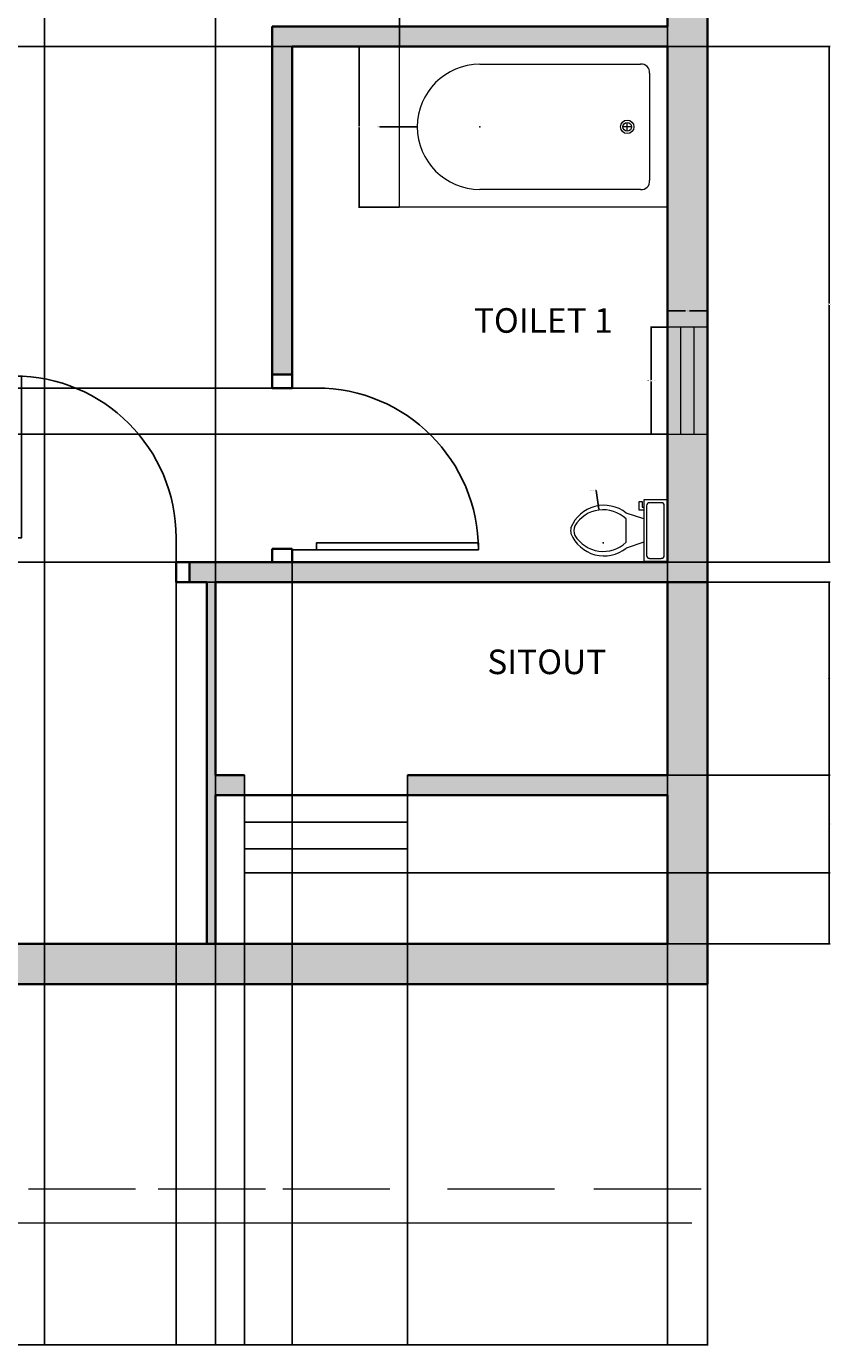
# Model space of a CAD drawing. Units: inches. Extents: x 1839 to 2285, y 722 to 1311.
# Tile 3 of 7: x 2105 to 2285, y 722 to 1018. Entities that reach past the tile are written whole.
import ezdxf

# ---------------------------------------------------------------- set-up
doc = ezdxf.new("R2010")
doc.units = ezdxf.units.IN
for name, color, linetype, lineweight in [('A-ANNO-DIMS', 2, 'Continuous', 18), ('A-AREA-IDEN', 7, 'Continuous', 18), ('A-DOOR', 3, 'Continuous', 25), ('A-FLOR-FIXT', 9, 'Continuous', 18), ('A-FLOR-STRS', 7, 'Continuous', 25), ('A-GLAZ', 4, 'Continuous', 18), ('A-GLAZ-PATT', 9, 'Continuous', 13), ('A-WALL', 7, 'Continuous', 35), ('C-ROAD', 8, 'Continuous', 18)]:
    doc.layers.add(name, color=color, linetype=linetype, lineweight=lineweight)
doc.layers.add('A-WALL-PATT', color=18, linetype='Continuous', lineweight=13, true_color=0x000000)
doc.styles.get("Standard").update_dxf_attribs({"font": 'arial.ttf'})
doc.dimstyles.get("Standard").update_dxf_attribs({"dimtxt": 0.18, "dimasz": 0.18, "dimexe": 0.18, "dimexo": 0.0625, "dimgap": 0.09, "dimtad": 0, "dimtih": 1, "dimtoh": 1, "dimdec": 4, "dimzin": 0, "dimdsep": 46, "dimtxsty": 'Standard', "dimcen": 0.09, "dimadec": 0, "dimazin": 0, "dimtfac": 1, "dimtdec": 4, "dimtofl": 0, "dimtmove": 0, "dimatfit": 3, "dimfxl": 1, "dimtolj": 1, "dimtzin": 0, "dimarcsym": 0})

# ---------------------------------------------------------------- blocks, each defined once
blk = doc.blocks.new('*U3')
for p, q in [((0, 0), (0, -6)), ((-40, 0), (-40, -6))]:
    blk.add_line(p, q)
blk.add_lwpolyline([(0, 0), (0, 40), (-1.75, 40), (-1.75, 0)], close=True)
blk.add_arc((0, 0), 40, 90, 180)
blk = doc.blocks.new('*U5')
for p, q in [((0, 0), (0, -6)), ((40, 0), (40, -6))]:
    blk.add_line(p, q)
blk.add_lwpolyline([(0, 0), (0, 40), (1.75, 40), (1.75, 0)], close=True)
blk.add_arc((0, 0), 40, 0, 90)
blk = doc.blocks.new('Toilet - top')
for p, q in [((9.5, -6), (9.5, -2)), ((-10, -8.5), (-8, -8.5)), ((-10, -9.5), (-10, -8.5)), ((-8, -8.5), (-8, -8)), ((-7, -8), (-7, -9.5)), ((-4, -8), (-6, -14)), ((4, -8), (6, -14)), ((-7, -9.5), (-10, -9.5)), ((4, -14), (-4, -14))]:
    blk.add_line(p, q)
blk.add_lwpolyline([(10.5, -8), (10.5, 0), (-10.5, 0), (-10.5, -8)], close=True)
for points in [[(-9.5, -2), (-9.5, -6)], [(8.5, -1), (-8.5, -1)], [(-8.5, -7), (8.5, -7)]]:
    blk.add_lwpolyline(points)
for centre, radius, start, end in [((-8.62, -1.88), 0.884, 81.8699, 188.1301), ((8.62, -1.88), 0.884, 351.8699, 98.1301), ((-8.62, -6.12), 0.884, 171.8699, 278.1301), ((8.62, -6.12), 0.884, 261.8699, 8.1301), ((3.52, -21.58), 12.17, 141.4691, 247.9714), ((4.2, -21.82), 11.33, 136.3677, 238.9468), ((-3.52, -21.58), 12.17, 292.0284, 38.5307), ((-4.2, -21.82), 11.33, 301.053, 43.6321), ((0, -27.88), 4, 245.7318, 294.2682), ((0, -29), 4, 254.8605, 285.1395)]:
    blk.add_arc(centre, radius, start, end)
blk = doc.blocks.new('Bath Tub - 26 x 60 in.')
for p, q in [((9, -17), (9, -19)), ((8, -18), (10, -18))]:
    blk.add_line(p, q)
blk.add_lwpolyline([(0, -36), (0, 0), (60, 0), (60, -36)], close=True)
for points in [[(6, -4), (42, -4)], [(4, -30), (4, -6)], [(42, -32), (6, -32)]]:
    blk.add_lwpolyline(points)
for radius in [1.5, 1]:
    blk.add_circle((9, -18), radius)
for centre, radius, start, end in [((5.75, -5.75), 1.77, 81.8699, 188.1301), ((42, -18), 14, 270, 90), ((5.75, -30.25), 1.77, 171.8699, 278.1301)]:
    blk.add_arc(centre, radius, start, end)
blk = doc.blocks.new('WIN-24x9')
for p, q in [((3, 0), (3, 24)), ((6, 0), (6, 24))]:
    blk.add_line(p, q)
blk.add_lwpolyline([(0, 24), (0, 0), (9, 0), (9, 24)], close=True)
blk = doc.blocks.new('*D21')
at = {"layer": 'A-ANNO-DIMS', "color": 0, "lineweight": -2, "transparency": 16777216}
for p, q in [((2248.61, 950.49), (2244.9, 950.49)), ((2245.08, 950.31), (2245.08, 938.67)), ((2245.08, 926.67), (2245.08, 938.3)), ((2248.61, 926.49), (2244.9, 926.49))]:
    blk.add_line(p, q, dxfattribs=at)
at = {"layer": 'A-ANNO-DIMS', "color": 0, "transparency": 16777216}
for points in [[(2245.05, 950.31), (2245.11, 950.31), (2245.08, 950.49)], [(2245.05, 926.67), (2245.11, 926.67), (2245.08, 926.49)]]:
    blk.add_solid(points, dxfattribs=at)
at = {"layer": 'Defpoints', "color": 0, "transparency": 16777216}
for p in [(2245.08, 950.49), (2248.68, 950.49), (2248.68, 926.49)]:
    blk.add_point(p, dxfattribs=at)
at = {"layer": 'A-ANNO-DIMS', "color": 0, "transparency": 16777216, "insert": (2245.08, 938.49), "char_height": 0.18, "attachment_point": 5}
blk.add_mtext('\\A1;WINDOW 24 TYP.', dxfattribs=at)
blk = doc.blocks.new('*D22')
at = {"layer": 'A-ANNO-DIMS', "color": 0, "lineweight": -2, "transparency": 16777216}
for p, q in [((2248.68, 950.55), (2248.68, 954.27)), ((2248.86, 954.09), (2252.72, 954.09)), ((2257.5, 954.09), (2253.64, 954.09)), ((2257.68, 950.55), (2257.68, 954.27))]:
    blk.add_line(p, q, dxfattribs=at)
at = {"layer": 'A-ANNO-DIMS', "color": 0, "transparency": 16777216}
for points in [[(2248.86, 954.12), (2248.86, 954.06), (2248.68, 954.09)], [(2257.5, 954.12), (2257.5, 954.06), (2257.68, 954.09)]]:
    blk.add_solid(points, dxfattribs=at)
at = {"layer": 'Defpoints', "color": 0, "transparency": 16777216}
for p in [(2257.68, 954.09), (2248.68, 950.49), (2257.68, 950.49)]:
    blk.add_point(p, dxfattribs=at)
at = {"layer": 'A-ANNO-DIMS', "color": 0, "transparency": 16777216, "insert": (2253.18, 954.09), "char_height": 0.18, "attachment_point": 5}
blk.add_mtext('\\A1;9 TYP.', dxfattribs=at)
blk = doc.blocks.new('*D37')
at = {"layer": 'A-ANNO-DIMS', "color": 0, "lineweight": -2, "transparency": 16777216}
for p, q in [((2188.68, 1013.39), (2188.68, 1022.51)), ((2248.68, 1013.39), (2248.68, 1022.51)), ((2188.86, 1022.33), (2218.17, 1022.33)), ((2248.5, 1022.33), (2219.18, 1022.33))]:
    blk.add_line(p, q, dxfattribs=at)
at = {"layer": 'A-ANNO-DIMS', "color": 0, "transparency": 16777216}
for points in [[(2188.86, 1022.36), (2188.86, 1022.3), (2188.68, 1022.33)], [(2248.5, 1022.36), (2248.5, 1022.3), (2248.68, 1022.33)]]:
    blk.add_solid(points, dxfattribs=at)
at = {"layer": 'Defpoints', "color": 0, "transparency": 16777216}
for p in [(2188.68, 1022.33), (2188.68, 1013.33), (2248.68, 1013.33)]:
    blk.add_point(p, dxfattribs=at)
at = {"layer": 'A-ANNO-DIMS', "color": 0, "transparency": 16777216, "insert": (2218.68, 1022.33), "char_height": 0.18, "attachment_point": 5}
blk.add_mtext('\\A1;TUB 60', dxfattribs=at)
blk = doc.blocks.new('*D38')
at = {"layer": 'A-ANNO-DIMS', "color": 0, "lineweight": -2, "transparency": 16777216}
for p, q in [((2188.61, 1013.33), (2179.5, 1013.33)), ((2179.68, 1013.15), (2179.68, 995.51)), ((2179.68, 977.51), (2179.68, 995.15)), ((2188.61, 977.33), (2179.5, 977.33))]:
    blk.add_line(p, q, dxfattribs=at)
at = {"layer": 'A-ANNO-DIMS', "color": 0, "transparency": 16777216}
for points in [[(2179.65, 1013.15), (2179.71, 1013.15), (2179.68, 1013.33)], [(2179.65, 977.51), (2179.71, 977.51), (2179.68, 977.33)]]:
    blk.add_solid(points, dxfattribs=at)
at = {"layer": 'Defpoints', "color": 0, "transparency": 16777216}
for p in [(2188.68, 1013.33), (2179.68, 977.33), (2188.68, 977.33)]:
    blk.add_point(p, dxfattribs=at)
at = {"layer": 'A-ANNO-DIMS', "color": 0, "transparency": 16777216, "insert": (2179.68, 995.33), "char_height": 0.18, "attachment_point": 5}
blk.add_mtext('\\A1;36', dxfattribs=at)
blk = doc.blocks.new('*D41')
at = {"layer": 'A-ANNO-DIMS', "color": 0, "lineweight": -2, "transparency": 16777216}
for p, q in [((1897.68, 803.27), (1897.68, 722.34)), ((2257.68, 803.27), (2257.68, 722.34)), ((1897.86, 722.52), (2077.39, 722.52)), ((2257.5, 722.52), (2077.97, 722.52))]:
    blk.add_line(p, q, dxfattribs=at)
at = {"layer": 'A-ANNO-DIMS', "color": 0, "transparency": 16777216}
for points in [[(1897.86, 722.55), (1897.86, 722.49), (1897.68, 722.52)], [(2257.5, 722.55), (2257.5, 722.49), (2257.68, 722.52)]]:
    blk.add_solid(points, dxfattribs=at)
at = {"layer": 'Defpoints', "color": 0, "transparency": 16777216}
for p in [(1897.68, 803.33), (2257.68, 803.33), (2257.68, 722.52)]:
    blk.add_point(p, dxfattribs=at)
at = {"layer": 'A-ANNO-DIMS', "color": 0, "transparency": 16777216, "insert": (2077.68, 722.52), "char_height": 0.18, "attachment_point": 5}
blk.add_mtext('\\A1;360', dxfattribs=at)
blk = doc.blocks.new('*D45')
at = {"layer": 'A-ANNO-DIMS', "color": 0, "lineweight": -2, "transparency": 16777216}
for p, q in [((2109.18, 1145.02), (2109.18, 722.34)), ((2248.68, 1142.27), (2248.68, 722.34)), ((2109.36, 722.52), (2178.54, 722.52)), ((2248.5, 722.52), (2179.31, 722.52))]:
    blk.add_line(p, q, dxfattribs=at)
at = {"layer": 'A-ANNO-DIMS', "color": 0, "transparency": 16777216}
for points in [[(2109.36, 722.55), (2109.36, 722.49), (2109.18, 722.52)], [(2248.5, 722.55), (2248.5, 722.49), (2248.68, 722.52)]]:
    blk.add_solid(points, dxfattribs=at)
at = {"layer": 'Defpoints', "color": 0, "transparency": 16777216}
for p in [(2109.18, 1145.08), (2248.68, 1142.33), (2248.68, 722.52)]:
    blk.add_point(p, dxfattribs=at)
at = {"layer": 'A-ANNO-DIMS', "color": 0, "transparency": 16777216, "insert": (2178.93, 722.52), "char_height": 0.18, "attachment_point": 5}
blk.add_mtext('\\A1;139.5', dxfattribs=at)
blk = doc.blocks.new('*D49')
at = {"layer": 'A-ANNO-DIMS', "color": 0, "lineweight": -2, "transparency": 16777216}
for p, q in [((2248.74, 1013.33), (2285.11, 1013.33)), ((2284.93, 1013.15), (2284.93, 955.76)), ((2284.93, 898.01), (2284.93, 955.4)), ((2248.74, 897.83), (2285.11, 897.83))]:
    blk.add_line(p, q, dxfattribs=at)
at = {"layer": 'A-ANNO-DIMS', "color": 0, "transparency": 16777216}
for points in [[(2284.9, 1013.15), (2284.96, 1013.15), (2284.93, 1013.33)], [(2284.9, 898.01), (2284.96, 898.01), (2284.93, 897.83)]]:
    blk.add_solid(points, dxfattribs=at)
at = {"layer": 'Defpoints', "color": 0, "transparency": 16777216}
for p in [(2248.68, 1013.33), (2284.93, 1013.33), (2248.68, 897.83)]:
    blk.add_point(p, dxfattribs=at)
at = {"layer": 'A-ANNO-DIMS', "color": 0, "transparency": 16777216, "insert": (2284.93, 955.58), "char_height": 0.18, "attachment_point": 5}
blk.add_mtext('\\A1;115.5', dxfattribs=at)
blk = doc.blocks.new('*D50')
at = {"layer": 'A-ANNO-DIMS', "color": 0, "lineweight": -2, "transparency": 16777216}
for p, q in [((2145.57, 893.33), (2285.11, 893.33)), ((2284.93, 893.15), (2284.93, 853.01)), ((2284.93, 812.51), (2284.93, 852.65)), ((1906.74, 812.33), (2285.11, 812.33))]:
    blk.add_line(p, q, dxfattribs=at)
at = {"layer": 'A-ANNO-DIMS', "color": 0, "transparency": 16777216}
for points in [[(2284.9, 893.15), (2284.96, 893.15), (2284.93, 893.33)], [(2284.9, 812.51), (2284.96, 812.51), (2284.93, 812.33)]]:
    blk.add_solid(points, dxfattribs=at)
at = {"layer": 'Defpoints', "color": 0, "transparency": 16777216}
for p in [(2145.5, 893.33), (2284.93, 893.33), (1906.68, 812.33)]:
    blk.add_point(p, dxfattribs=at)
at = {"layer": 'A-ANNO-DIMS', "color": 0, "transparency": 16777216, "insert": (2284.93, 852.83), "char_height": 0.18, "attachment_point": 5}
blk.add_mtext('\\A1;81', dxfattribs=at)
blk = doc.blocks.new('*D54')
at = {"layer": 'A-ANNO-DIMS', "color": 0, "lineweight": -2, "transparency": 16777216}
for p, q in [((2164.68, 897.77), (2164.68, 722.34)), ((2248.68, 897.77), (2248.68, 722.34)), ((2164.86, 722.52), (2206.46, 722.52)), ((2248.5, 722.52), (2206.9, 722.52))]:
    blk.add_line(p, q, dxfattribs=at)
at = {"layer": 'A-ANNO-DIMS', "color": 0, "transparency": 16777216}
for points in [[(2164.86, 722.55), (2164.86, 722.49), (2164.68, 722.52)], [(2248.5, 722.55), (2248.5, 722.49), (2248.68, 722.52)]]:
    blk.add_solid(points, dxfattribs=at)
at = {"layer": 'Defpoints', "color": 0, "transparency": 16777216}
for p in [(2164.68, 897.83), (2248.68, 897.83), (2248.68, 722.52)]:
    blk.add_point(p, dxfattribs=at)
at = {"layer": 'A-ANNO-DIMS', "color": 0, "transparency": 16777216, "insert": (2206.68, 722.52), "char_height": 0.18, "attachment_point": 5}
blk.add_mtext('\\A1;84', dxfattribs=at)
blk = doc.blocks.new('*D56')
at = {"layer": 'A-ANNO-DIMS', "color": 0, "lineweight": -2, "transparency": 16777216}
for p, q in [((2147.5, 850.18), (2147.5, 1310.76)), ((2147.68, 1310.58), (2197.64, 1310.58)), ((2248.5, 1310.58), (2198.55, 1310.58)), ((2248.68, 850.18), (2248.68, 1310.76))]:
    blk.add_line(p, q, dxfattribs=at)
at = {"layer": 'A-ANNO-DIMS', "color": 0, "transparency": 16777216}
for points in [[(2147.68, 1310.61), (2147.68, 1310.55), (2147.5, 1310.58)], [(2248.5, 1310.61), (2248.5, 1310.55), (2248.68, 1310.58)]]:
    blk.add_solid(points, dxfattribs=at)
at = {"layer": 'Defpoints', "color": 0, "transparency": 16777216}
for p in [(2248.68, 1310.58), (2147.5, 850.11), (2248.68, 850.11)]:
    blk.add_point(p, dxfattribs=at)
at = {"layer": 'A-ANNO-DIMS', "color": 0, "transparency": 16777216, "insert": (2198.09, 1310.58), "char_height": 0.18, "attachment_point": 5}
blk.add_mtext('\\A1;101.17', dxfattribs=at)
blk = doc.blocks.new('*D57')
at = {"layer": 'A-ANNO-DIMS', "color": 0, "lineweight": -2, "transparency": 16777216}
for p, q in [((2248.74, 893.33), (2285.11, 893.33)), ((2284.93, 893.15), (2284.93, 871.9)), ((2284.93, 850.29), (2284.93, 871.54)), ((2248.74, 850.11), (2285.11, 850.11))]:
    blk.add_line(p, q, dxfattribs=at)
at = {"layer": 'A-ANNO-DIMS', "color": 0, "transparency": 16777216}
for points in [[(2284.9, 893.15), (2284.96, 893.15), (2284.93, 893.33)], [(2284.9, 850.29), (2284.96, 850.29), (2284.93, 850.11)]]:
    blk.add_solid(points, dxfattribs=at)
at = {"layer": 'Defpoints', "color": 0, "transparency": 16777216}
for p in [(2248.68, 893.33), (2284.93, 893.33), (2248.68, 850.11)]:
    blk.add_point(p, dxfattribs=at)
at = {"layer": 'A-ANNO-DIMS', "color": 0, "transparency": 16777216, "insert": (2284.93, 871.72), "char_height": 0.18, "attachment_point": 5}
blk.add_mtext('\\A1;43.22', dxfattribs=at)
blk = doc.blocks.new('*D58')
at = {"layer": 'A-ANNO-DIMS', "color": 0, "lineweight": -2, "transparency": 16777216}
for p, q in [((2102.66, 893.27), (2102.66, 722.34)), ((2138.66, 893.27), (2138.66, 722.34)), ((2102.84, 722.52), (2120.45, 722.52)), ((2138.48, 722.52), (2120.88, 722.52))]:
    blk.add_line(p, q, dxfattribs=at)
at = {"layer": 'A-ANNO-DIMS', "color": 0, "transparency": 16777216}
for points in [[(2102.84, 722.55), (2102.84, 722.49), (2102.66, 722.52)], [(2138.48, 722.55), (2138.48, 722.49), (2138.66, 722.52)]]:
    blk.add_solid(points, dxfattribs=at)
at = {"layer": 'Defpoints', "color": 0, "transparency": 16777216}
for p in [(2102.66, 893.33), (2138.66, 893.33), (2138.66, 722.52)]:
    blk.add_point(p, dxfattribs=at)
at = {"layer": 'A-ANNO-DIMS', "color": 0, "transparency": 16777216, "insert": (2120.66, 722.52), "char_height": 0.18, "attachment_point": 5}
blk.add_mtext('\\A1;36', dxfattribs=at)
blk = doc.blocks.new('*D64')
at = {"layer": 'A-ANNO-DIMS', "color": 0, "lineweight": -2, "transparency": 16777216}
for p, q in [((2248.61, 926.49), (1870.25, 926.49)), ((1870.43, 926.31), (1870.43, 912.34)), ((1870.43, 898.01), (1870.43, 911.98)), ((2248.61, 897.83), (1870.25, 897.83))]:
    blk.add_line(p, q, dxfattribs=at)
at = {"layer": 'A-ANNO-DIMS', "color": 0, "transparency": 16777216}
for points in [[(1870.4, 926.31), (1870.46, 926.31), (1870.43, 926.49)], [(1870.4, 898.01), (1870.46, 898.01), (1870.43, 897.83)]]:
    blk.add_solid(points, dxfattribs=at)
at = {"layer": 'Defpoints', "color": 0, "transparency": 16777216}
for p in [(1870.43, 926.49), (2248.68, 926.49), (2248.68, 897.83)]:
    blk.add_point(p, dxfattribs=at)
at = {"layer": 'A-ANNO-DIMS', "color": 0, "transparency": 16777216, "insert": (1870.43, 912.16), "char_height": 0.18, "attachment_point": 5}
blk.add_mtext('\\A1;28.655', dxfattribs=at)
blk = doc.blocks.new('*D76')
at = {"layer": 'A-ANNO-DIMS', "color": 0, "lineweight": -2, "transparency": 16777216}
for p, q in [((2153.99, 828.2), (2153.99, 722.34)), ((2190.49, 828.2), (2190.49, 722.34)), ((2154.17, 722.52), (2171.91, 722.52)), ((2190.31, 722.52), (2172.56, 722.52))]:
    blk.add_line(p, q, dxfattribs=at)
at = {"layer": 'A-ANNO-DIMS', "color": 0, "transparency": 16777216}
for points in [[(2154.17, 722.55), (2154.17, 722.49), (2153.99, 722.52)], [(2190.31, 722.55), (2190.31, 722.49), (2190.49, 722.52)]]:
    blk.add_solid(points, dxfattribs=at)
at = {"layer": 'Defpoints', "color": 0, "transparency": 16777216}
for p in [(2153.99, 828.26), (2190.49, 828.26), (2190.49, 722.52)]:
    blk.add_point(p, dxfattribs=at)
at = {"layer": 'A-ANNO-DIMS', "color": 0, "transparency": 16777216, "insert": (2172.24, 722.52), "char_height": 0.18, "attachment_point": 5}
blk.add_mtext('\\A1;36.5', dxfattribs=at)
blk = doc.blocks.new('*D77')
at = {"layer": 'A-ANNO-DIMS', "color": 0, "lineweight": -2, "transparency": 16777216}
for p, q in [((2190.55, 850.11), (2285.11, 850.11)), ((2284.93, 849.93), (2284.93, 839.37)), ((2284.93, 828.44), (2284.93, 839.01)), ((2190.55, 828.26), (2285.11, 828.26))]:
    blk.add_line(p, q, dxfattribs=at)
at = {"layer": 'A-ANNO-DIMS', "color": 0, "transparency": 16777216}
for points in [[(2284.9, 849.93), (2284.96, 849.93), (2284.93, 850.11)], [(2284.9, 828.44), (2284.96, 828.44), (2284.93, 828.26)]]:
    blk.add_solid(points, dxfattribs=at)
at = {"layer": 'Defpoints', "color": 0, "transparency": 16777216}
for p in [(2190.49, 850.11), (2284.93, 850.11), (2190.49, 828.26)]:
    blk.add_point(p, dxfattribs=at)
at = {"layer": 'A-ANNO-DIMS', "color": 0, "transparency": 16777216, "insert": (2284.93, 839.19), "char_height": 0.18, "attachment_point": 5}
blk.add_mtext('\\A1;21.85', dxfattribs=at)
blk = doc.blocks.new('*D80')
at = {"layer": 'A-ANNO-DIMS', "color": 0, "lineweight": -2, "transparency": 16777216}
for p, q in [((2147.5, 850.05), (2147.5, 722.34)), ((2153.99, 850.05), (2153.99, 722.34)), ((2147.68, 722.52), (2150.35, 722.52)), ((2153.81, 722.52), (2151.14, 722.52))]:
    blk.add_line(p, q, dxfattribs=at)
at = {"layer": 'A-ANNO-DIMS', "color": 0, "transparency": 16777216}
for points in [[(2147.68, 722.55), (2147.68, 722.49), (2147.5, 722.52)], [(2153.81, 722.55), (2153.81, 722.49), (2153.99, 722.52)]]:
    blk.add_solid(points, dxfattribs=at)
at = {"layer": 'Defpoints', "color": 0, "transparency": 16777216}
for p in [(2147.5, 850.11), (2153.99, 850.11), (2153.99, 722.52)]:
    blk.add_point(p, dxfattribs=at)
at = {"layer": 'A-ANNO-DIMS', "color": 0, "transparency": 16777216, "insert": (2150.74, 722.52), "char_height": 0.18, "attachment_point": 5}
blk.add_mtext('\\A1;6.482', dxfattribs=at)
blk = doc.blocks.new('*D82')
at = {"layer": 'A-ANNO-DIMS', "color": 0, "lineweight": -2, "transparency": 16777216}
for p, q in [((2164.61, 1013.33), (1870.25, 1013.33)), ((1870.43, 1013.15), (1870.43, 975.26)), ((1870.43, 937.01), (1870.43, 974.9)), ((2164.61, 936.83), (1870.25, 936.83))]:
    blk.add_line(p, q, dxfattribs=at)
at = {"layer": 'A-ANNO-DIMS', "color": 0, "transparency": 16777216}
for points in [[(1870.4, 1013.15), (1870.46, 1013.15), (1870.43, 1013.33)], [(1870.4, 937.01), (1870.46, 937.01), (1870.43, 936.83)]]:
    blk.add_solid(points, dxfattribs=at)
at = {"layer": 'Defpoints', "color": 0, "transparency": 16777216}
for p in [(1870.43, 1013.33), (2164.68, 1013.33), (2164.68, 936.83)]:
    blk.add_point(p, dxfattribs=at)
at = {"layer": 'A-ANNO-DIMS', "color": 0, "transparency": 16777216, "insert": (1870.43, 975.08), "char_height": 0.18, "attachment_point": 5}
blk.add_mtext('\\A1;76.5', dxfattribs=at)
blk = doc.blocks.new('*D85')
at = {"layer": 'A-ANNO-DIMS', "color": 0, "lineweight": -2, "transparency": 16777216}
for p, q in [((2184.28, 995.33), (2192.5, 995.33)), ((2206.59, 995.33), (2206.77, 995.33)), ((2206.68, 995.24), (2206.68, 995.42))]:
    blk.add_line(p, q, dxfattribs=at)
at = {"layer": 'A-ANNO-DIMS', "color": 0, "transparency": 16777216}
blk.add_solid([(2192.5, 995.36), (2192.5, 995.3), (2192.68, 995.33)], dxfattribs=at)
at = {"layer": 'Defpoints', "color": 0, "transparency": 16777216}
for p in [(2192.68, 995.33), (2206.68, 995.33)]:
    blk.add_point(p, dxfattribs=at)
at = {"layer": 'A-ANNO-DIMS', "color": 0, "transparency": 16777216, "insert": (2183.97, 995.33), "char_height": 0.18, "attachment_point": 5}
blk.add_mtext('\\A1;R14', dxfattribs=at)
blk = doc.blocks.new('*D92')
at = {"layer": 'A-ANNO-DIMS', "color": 0, "lineweight": -2, "transparency": 16777216}
for p, q in [((2232.56, 913.91), (2232.74, 913.91)), ((2232.74, 913.91), (2233.31, 909.68)), ((2234.23, 902.15), (2234.41, 902.15)), ((2234.32, 902.06), (2234.32, 902.24))]:
    blk.add_line(p, q, dxfattribs=at)
at = {"layer": 'A-ANNO-DIMS', "color": 0, "transparency": 16777216}
blk.add_solid([(2233.34, 909.68), (2233.28, 909.67), (2233.33, 909.5)], dxfattribs=at)
at = {"layer": 'Defpoints', "color": 0, "transparency": 16777216}
for p in [(2233.33, 909.5), (2234.32, 902.15)]:
    blk.add_point(p, dxfattribs=at)
at = {"layer": 'A-ANNO-DIMS', "color": 0, "transparency": 16777216, "insert": (2231.88, 913.91), "char_height": 0.18, "attachment_point": 5}
blk.add_mtext('\\A1;4X R7.419', dxfattribs=at)

msp = doc.modelspace()

# ---------------------------------------------------------------- hatches: boundary and pattern name
at = {"layer": 'A-GLAZ-PATT'}
h = msp.add_hatch(color=256, dxfattribs=at)
h.dxf.hatch_style = 1
h.set_gradient(color1=(0, 0, 255), color2=(255, 255, 0))
h.paths.add_polyline_path([(2251.6771, 950.4862), (2248.6771, 950.4862), (2248.6771, 926.4862), (2251.6771, 926.4862)])
h.paths.add_polyline_path([(2254.6771, 950.4862), (2251.6771, 950.4862), (2251.6771, 926.4862), (2254.6771, 926.4862)])
h.paths.add_polyline_path([(2257.6771, 950.4862), (2254.6771, 950.4862), (2254.6771, 926.4862), (2257.6771, 926.4862)])
at = {"layer": 'A-WALL-PATT'}
h = msp.add_hatch(color=256, dxfattribs=at)
h.dxf.hatch_style = 1
h.paths.add_polyline_path([(1906.6771, 1274.3314), (1942.6771, 1274.3314), (1942.6771, 1283.3314), (1897.6771, 1283.3314), (1897.6771, 968.2107), (1906.6771, 968.2107), (1906.6771, 1013.3314), (1939.6771, 1013.3314), (1939.6771, 1017.8314), (1906.6771, 1017.8314), (1906.6771, 1137.8314), (2050.6771, 1137.8314), (2050.6771, 1142.3314), (1906.6771, 1142.3314)])
h.paths.add_polyline_path([(2064.0508, 1283.3314), (1978.6771, 1283.3314), (1978.6771, 1274.3314), (2050.6771, 1274.3314), (2050.6771, 1184.3314), (2055.1771, 1184.3314), (2055.1771, 1214.3314), (2058.1771, 1214.3314), (2058.1771, 1218.8314), (2055.1771, 1218.8314), (2055.1771, 1274.3314), (2064.0508, 1274.3314)])
h.paths.add_polyline_path([(2182.6416, 1283.3314), (2088.0508, 1283.3314), (2088.0508, 1274.3314), (2104.6771, 1274.3314), (2104.6771, 1218.8314), (2094.1771, 1218.8314), (2094.1771, 1214.3314), (2104.6771, 1214.3314), (2104.6771, 1184.3314), (2109.1771, 1184.3314), (2109.1771, 1274.3314), (2182.6416, 1274.3314)])
h.paths.add_polyline_path([(2257.6771, 1283.3314), (2218.6416, 1283.3314), (2218.6416, 1274.3314), (2248.6771, 1274.3314), (2248.6771, 1142.3314), (2186.4004, 1142.3314), (2109.1771, 1142.3314), (2109.1771, 1137.8314), (2248.6771, 1137.8314), (2248.6771, 1094.9086), (2257.6771, 1094.9086)])
h.paths.add_polyline_path([(2257.6771, 1058.9086), (2248.6771, 1058.9086), (2248.6771, 1017.8314), (2160.1771, 1017.8314), (2160.1771, 939.8314), (2164.6771, 939.8314), (2164.6771, 1013.3314), (2248.6771, 1013.3314), (2248.6771, 977.3314), (2248.6771, 950.4862), (2257.6771, 950.4862)])
h.paths.add_polyline_path([(2257.6771, 893.3314), (2248.6771, 893.3314), (2248.6771, 850.1143), (2190.4862, 850.1143), (2190.4862, 845.6143), (2248.6771, 845.6143), (2248.6771, 812.3314), (2100.5038, 812.3314), (2100.5038, 803.3314), (2257.6771, 803.3314)])
h.paths.add_polyline_path([(2257.6771, 926.4862), (2248.6771, 926.4862), (2248.6771, 897.8314), (2141.6642, 897.8314), (2141.6642, 893.3314), (2145.5038, 893.3314), (2145.5038, 812.3314), (2147.5038, 812.3314), (2147.5038, 845.6143), (2153.9854, 845.6143), (2153.9854, 850.1143), (2147.5038, 850.1143), (2147.5038, 893.3314), (2248.6771, 893.3314), (2257.6771, 893.3314)])
h.paths.add_polyline_path([(1906.6771, 893.3314), (1897.6771, 893.3314), (1897.6771, 803.3314), (2022.5038, 803.3314), (2022.5038, 812.3314), (1906.6771, 812.3314)])
h.paths.add_polyline_path([(2031.4676, 897.8314), (1981.6771, 897.8314), (1981.6771, 1013.3314), (2024.6642, 1013.3314), (2024.6642, 1017.8314), (1975.6771, 1017.8314), (1975.6771, 1013.3314), (1978.6771, 1013.3314), (1978.6771, 897.8314), (1906.6771, 897.8314), (1906.6771, 932.2107), (1897.6771, 932.2107), (1897.6771, 893.3314), (1906.6771, 893.3314), (2031.4676, 893.3314)])
h.paths.add_polyline_path([(2099.6642, 1017.8314), (2096.6642, 1017.8314), (2084.1956, 1017.8314), (2084.1956, 1013.3314), (2096.6642, 1013.3314), (2096.6642, 897.8314), (2085.6129, 897.8314), (2085.6129, 893.3314), (2102.6642, 893.3314), (2102.6642, 897.8314), (2099.6642, 897.8314)])

# ---------------------------------------------------------------- linework, layer by layer
at = {"layer": 'A-FLOR-STRS'}
for p, q in [((2153.9854, 828.2621), (2153.9854, 850.1143)), ((2190.4862, 850.1143), (2190.4862, 828.2621)), ((2153.9854, 839.6143), (2190.4862, 839.6143)), ((2153.9854, 833.6143), (2190.4862, 833.6143)), ((2190.4862, 828.2621), (2153.9854, 828.2621))]:
    msp.add_line(p, q, dxfattribs=at)
at = {"layer": 'A-WALL'}
for p, q in [((2248.6771, 1137.8314), (2248.6771, 1017.8314)), ((2160.1771, 1017.8314), (2160.1771, 936.8314)), ((2160.1771, 1017.8314), (2248.6771, 1017.8314)), ((2164.6771, 1013.3314), (2164.6771, 936.8314)), ((2164.6771, 1013.3314), (2248.6771, 1013.3314)), ((2248.6771, 1013.3314), (2248.6771, 897.8314)), ((2160.1771, 939.8314), (2164.6771, 939.8314)), ((2160.1771, 936.8314), (2164.6771, 936.8314)), ((2160.1771, 900.8314), (2164.6771, 900.8314)), ((2160.1771, 900.8314), (2160.1771, 897.8314)), ((2164.6771, 900.8314), (2164.6771, 897.8314)), ((2138.6642, 893.3314), (2138.6642, 897.8314)), ((2138.6642, 897.8314), (2248.6771, 897.8314)), ((2141.6642, 893.3314), (2141.6642, 897.8314)), ((2138.6642, 893.3314), (2145.5038, 893.3314)), ((2145.5038, 893.3314), (2145.5038, 812.3314)), ((2147.5038, 893.3314), (2147.5038, 850.1143)), ((2147.5038, 893.3314), (2248.6771, 893.3314)), ((2248.6771, 893.3314), (2248.6771, 850.1143)), ((2248.6771, 893.3314), (2257.6771, 893.3314)), ((2147.5038, 850.1143), (2153.9854, 850.1143)), ((2190.4862, 850.1143), (2248.6771, 850.1143)), ((2147.5038, 845.6143), (2153.9854, 845.6143)), ((2147.5038, 845.6143), (2147.5038, 812.3314)), ((2153.9854, 845.6143), (2248.6771, 845.6143)), ((2248.6771, 845.6143), (2248.6771, 812.3314)), ((2248.6771, 812.3314), (2100.5038, 812.3314))]:
    msp.add_line(p, q, dxfattribs=at)
msp.add_lwpolyline([(2022.5038, 803.3314), (1897.6771, 803.3314), (1897.6771, 1283.3314), (2257.6771, 1283.3314), (2257.6771, 803.3314), (2100.5038, 803.3314)], dxfattribs=at)
at = {"layer": 'C-ROAD'}
for p, q in [((2105.5746, 757.4754), (2129.5746, 757.4754)), ((2134.645, 757.4754), (2158.645, 757.4754)), ((2162.5365, 757.4754), (2186.5365, 757.4754)), ((2199.3992, 757.4754), (2223.3992, 757.4754)), ((2232.2221, 757.4754), (2256.2221, 757.4754)), ((2254.1419, 749.766), (1899.596, 749.766))]:
    msp.add_line(p, q, dxfattribs=at)

# ---------------------------------------------------------------- block references
at = {"layer": 'A-DOOR', "xscale": 0.9062393225401889, "yscale": 0.9062393225401889, "zscale": 0.9062393225401889}
msp.add_blockref('*U5', (2102.4146, 903.2689), dxfattribs=at)
at = {"layer": 'A-DOOR', "xscale": 0.9062393225401889, "yscale": 0.9062393225401889, "zscale": 0.9062393225401889, "rotation": 270}
msp.add_blockref('*U3', (2170.1145, 900.5819), dxfattribs=at)
at = {"layer": 'A-FLOR-FIXT', "rotation": 180}
msp.add_blockref('Bath Tub - 26 x 60 in.', (2248.6771, 977.3314), dxfattribs=at)
at = {"layer": 'A-FLOR-FIXT', "xscale": 0.6548161329715463, "yscale": 0.6548161329715463, "zscale": 0.6548161329715463, "rotation": 270}
msp.add_blockref('Toilet - top', (2248.6069, 904.8979), dxfattribs=at)
at = {"layer": 'A-GLAZ'}
msp.add_blockref('WIN-24x9', (2248.677, 926.486), dxfattribs=at)

# ---------------------------------------------------------------- texts
at = {"layer": 'A-AREA-IDEN'}
for s, p in [('TOILET 1 ', (2205.3346, 949.2068)), ('SITOUT ', (2208.3484, 872.7424))]:
    msp.add_text(s, height=5.50379, dxfattribs=at).set_placement(p)

# ---------------------------------------------------------------- dimensions: what is measured, and where the dimension line sits
at = {"layer": 'A-ANNO-DIMS'}
for base, p1, p2, override, picture, middle in [((2248.6771, 1310.5814), (2147.5038, 850.1143), (2248.6771, 850.1143), {"dimdec": 2, "dimlfac": 1, "dimrnd": 0, "dimzin": 0, "dimdsep": 46, "dimlunit": 2}, '*D56', (2198.0905, 1310.5814)), ((2248.6771, 722.516), (2109.1771, 1145.0819), (2248.6771, 1142.3314), {"dimdec": 1, "dimlfac": 1, "dimrnd": 0, "dimzin": 0, "dimdsep": 46, "dimlunit": 2}, '*D45', (2178.9271, 722.516)), ((2248.6771, 722.516), (2164.6771, 897.8314), (2248.6771, 897.8314), {"dimdec": 0, "dimlfac": 1, "dimrnd": 0, "dimzin": 0, "dimdsep": 46, "dimlunit": 2}, '*D54', (2206.6771, 722.516)), ((2138.6642, 722.516), (2102.6642, 893.3314), (2138.6642, 893.3314), {"dimdec": 0, "dimlfac": 1, "dimrnd": 0, "dimzin": 0, "dimdsep": 46, "dimlunit": 2}, '*D58', (2120.6642, 722.516)), ((2153.9854, 722.516), (2147.5038, 850.1143), (2153.9854, 850.1143), {"dimdec": 3, "dimlfac": 1, "dimrnd": 0, "dimzin": 0, "dimdsep": 46, "dimlunit": 2}, '*D80', (2150.7446, 722.516)), ((2190.4862, 722.516), (2153.9854, 828.2621), (2190.4862, 828.2621), {"dimdec": 1, "dimlfac": 1, "dimrnd": 0, "dimzin": 0, "dimdsep": 46, "dimlunit": 2}, '*D76', (2172.2358, 722.516)), ((2257.6771, 722.516), (1897.6771, 803.3314), (2257.6771, 803.3314), {"dimdec": 0, "dimlfac": 1, "dimrnd": 0, "dimzin": 0, "dimdsep": 46, "dimlunit": 2}, '*D41', (2077.6771, 722.516))]:
    dim = msp.add_linear_dim(base=base, p1=p1, p2=p2, dimstyle='Standard', override=override, dxfattribs=at)
    dim.commit()
    dim.dimension.update_dxf_attribs({"geometry": picture, "text_midpoint": middle})
for base, p1, p2, angle, text, picture, middle in [((2188.6771, 1022.3314), (2248.6771, 1013.3314), (2188.6771, 1013.3314), 180, 'TUB <>', '*D37', (2218.6771, 1022.3314)), ((2245.0771, 950.4862), (2248.6771, 926.4862), (2248.6771, 950.4862), 90, 'WINDOW <> TYP.', '*D21', (2245.0771, 938.4862))]:
    dim = msp.add_linear_dim(base=base, p1=p1, p2=p2, angle=angle, text=text, dimstyle='Standard', override={"dimdec": 0, "dimlfac": 1, "dimrnd": 0, "dimzin": 0, "dimdsep": 46, "dimlunit": 2}, dxfattribs=at)
    dim.commit()
    dim.dimension.update_dxf_attribs({"geometry": picture, "text_midpoint": middle})
for base, p1, p2, angle, override, picture, middle in [((1870.4271, 1013.3314), (2164.6771, 936.8314), (2164.6771, 1013.3314), 90, {"dimdec": 1, "dimlfac": 1, "dimrnd": 0, "dimzin": 0, "dimdsep": 46, "dimlunit": 2}, '*D82', (1870.4271, 975.0814)), ((2179.6771, 977.3314), (2188.6771, 1013.3314), (2188.6771, 977.3314), 270, {"dimdec": 0, "dimlfac": 1, "dimrnd": 0, "dimzin": 0, "dimdsep": 46, "dimlunit": 2}, '*D38', (2179.6771, 995.3314)), ((2284.9271, 1013.3314), (2248.6771, 897.8314), (2248.6771, 1013.3314), 90, {"dimdec": 1, "dimlfac": 1, "dimrnd": 0, "dimzin": 0, "dimdsep": 46, "dimlunit": 2}, '*D49', (2284.9271, 955.5814)), ((1870.4271, 926.4862), (2248.6771, 897.8314), (2248.6771, 926.4862), 90, {"dimdec": 3, "dimlfac": 1, "dimrnd": 0, "dimzin": 0, "dimdsep": 46, "dimlunit": 2}, '*D64', (1870.4271, 912.1588)), ((2284.9271, 893.3314), (1906.6771, 812.3314), (2145.5038, 893.3314), 90, {"dimdec": 0, "dimlfac": 1, "dimrnd": 0, "dimzin": 0, "dimdsep": 46, "dimlunit": 2}, '*D50', (2284.9271, 852.8314)), ((2284.9271, 893.3314), (2248.6771, 850.1143), (2248.6771, 893.3314), 90, {"dimdec": 2, "dimlfac": 1, "dimrnd": 0, "dimzin": 0, "dimdsep": 46, "dimlunit": 2}, '*D57', (2284.9271, 871.7228)), ((2284.9271, 850.1143), (2190.4862, 828.2621), (2190.4862, 850.1143), 90, {"dimdec": 2, "dimlfac": 1, "dimrnd": 0, "dimzin": 0, "dimdsep": 46, "dimlunit": 2}, '*D77', (2284.9271, 839.1882))]:
    dim = msp.add_linear_dim(base=base, p1=p1, p2=p2, angle=angle, dimstyle='Standard', override=override, dxfattribs=at)
    dim.commit()
    dim.dimension.update_dxf_attribs({"geometry": picture, "text_midpoint": middle})
dim = msp.add_radius_dim(center=(2206.6771, 995.3314), mpoint=(2192.6771, 995.331), dimstyle='Standard', override={"dimdec": 0, "dimlfac": 1, "dimrnd": 0, "dimzin": 0, "dimdsep": 46, "dimlunit": 2}, dxfattribs=at)
dim.commit()
dim.dimension.update_dxf_attribs({"geometry": '*D85', "text_midpoint": (2184.2771, 995.3307), "dimtype": 164})
dim = msp.add_linear_dim(base=(2257.6771, 954.0862), p1=(2248.6771, 950.4862), p2=(2257.6771, 950.4862), text='<> TYP.', dimstyle='Standard', override={"dimdec": 0, "dimlfac": 1, "dimrnd": 0, "dimzin": 0, "dimdsep": 46, "dimlunit": 2}, dxfattribs=at)
dim.commit()
dim.dimension.update_dxf_attribs({"geometry": '*D22', "text_midpoint": (2253.1771, 954.0862)})
dim = msp.add_radius_dim(center=(2234.3205, 902.1477), mpoint=(2233.332, 909.5001), text='4X <>', dimstyle='Standard', override={"dimdec": 3, "dimlfac": 1, "dimrnd": 0, "dimzin": 0, "dimdsep": 46, "dimlunit": 2}, dxfattribs=at)
dim.commit()
dim.dimension.update_dxf_attribs({"geometry": '*D92', "text_midpoint": (2231.8819, 913.9115), "dimtype": 164})

doc.saveas('drawing.dxf')
